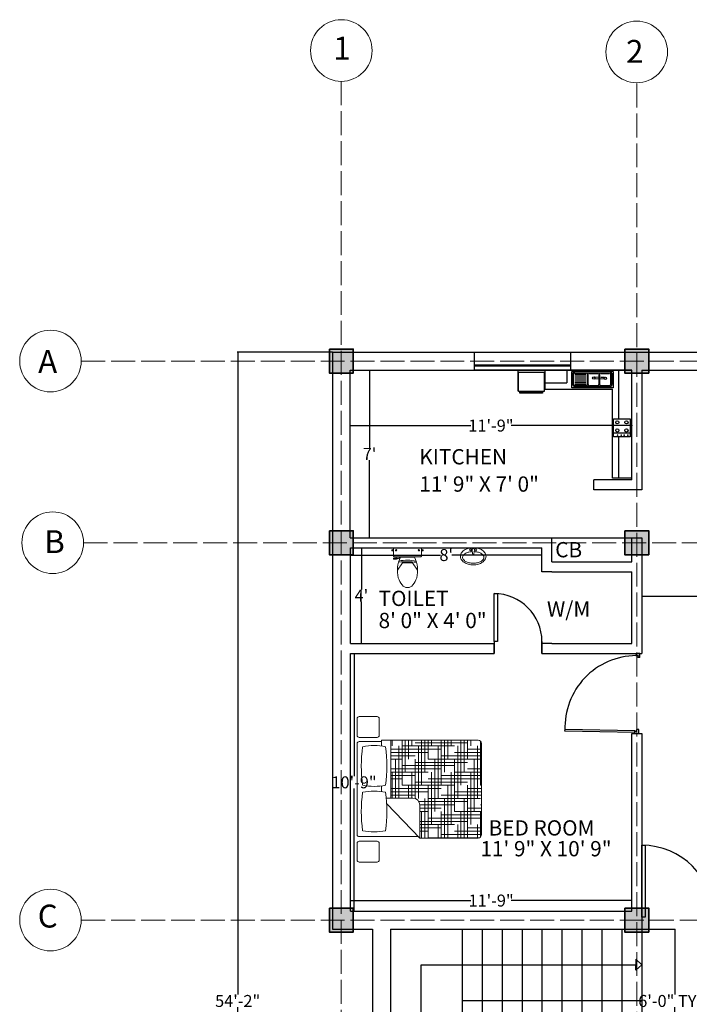
# Model space of a CAD drawing. Units: inches. Extents: x -113 to 5399, y -1393 to 3302.
# Tile 6 of 40: x 737 to 1073, y 460 to 953. Entities that reach past the tile are written whole.
import ezdxf

# ---------------------------------------------------------------- set-up
doc = ezdxf.new("R2010")
doc.units = ezdxf.units.IN
doc.header["$MEASUREMENT"] = 0
doc.linetypes.add('ACAD_ISO02W100', pattern=[15, 12, -3])
for name, color, linetype, lineweight in [('A-ANNO-DIMS', 254, 'Continuous', 18), ('A-AREA-IDEN', 4, 'Continuous', 18), ('A-COLS', 7, 'Continuous', 35), ('A-FLOR-CASE', 8, 'Continuous', 18), ('A-FLOR-FIXT', 8, 'Continuous', 18), ('A-GRID-IDEN', 7, 'Continuous', 18), ('doors', 2, 'Continuous', 25), ('DT TEXT', 4, 'Continuous', 18), ('furniture', 131, 'Continuous', 18), ('GRIDS', 7, 'ACAD_ISO02W100', 13), ('stairs', 210, 'Continuous', 25), ('walls', 1, 'Continuous', 25), ('windows', 3, 'Continuous', 25)]:
    doc.layers.add(name, color=color, linetype=linetype, lineweight=lineweight)
doc.layers.add('TEFRIŞ', color=11, linetype='Continuous')
doc.styles.get("Standard").update_dxf_attribs({"font": 'arial.ttf'})
doc.dimstyles.get("Standard").update_dxf_attribs({"dimtxt": 6, "dimasz": 0.18, "dimexe": 0.18, "dimexo": 0.0625, "dimgap": 0.09, "dimtad": 0, "dimtih": 1, "dimtoh": 1, "dimdec": 1, "dimzin": 0, "dimdsep": 46, "dimlunit": 4, "dimtxsty": 'Standard', "dimblk": 'ARCHTICK', "dimcen": 0.09, "dimadec": 0, "dimazin": 0, "dimtfac": 1, "dimtdec": 1, "dimtofl": 0, "dimtmove": 0, "dimatfit": 3, "dimfxl": 1, "dimtolj": 1, "dimtzin": 0, "dimarcsym": 0})

# ---------------------------------------------------------------- blocks, each defined once
blk = doc.blocks.new('*U2')
for p, q in [((0, 0), (0, -6)), ((24, 0), (24, -6))]:
    blk.add_line(p, q)
blk.add_lwpolyline([(0, 0), (0, 24), (1.75, 24), (1.75, 0)], close=True)
blk.add_arc((0, 0), 24, 0, 90)
blk = doc.blocks.new('*U3')
for p, q in [((0, 0), (0, -6)), ((36, 0), (36, -6))]:
    blk.add_line(p, q)
blk.add_lwpolyline([(0, 0), (0, 36), (1.75, 36), (1.75, 0)], close=True)
blk.add_arc((0, 0), 36, 0, 90)
blk = doc.blocks.new('*X4')
at = {"color": 0}
for p, q in [((4.359, 18.562), (4.359, 18.646)), ((4.5, 18), (4.5, 18.646)), ((4.547, 18.188), (4.547, 18.646)), ((4.594, 18.375), (4.594, 18.646)), ((4.641, 18.562), (4.641, 18.646)), ((4.687, 18.609), (5.437, 18.609)), ((4.781, 18), (4.781, 18.646)), ((4.828, 18.188), (4.828, 18.646)), ((4.875, 18.375), (4.875, 18.646)), ((4.922, 18.562), (4.922, 18.646)), ((5.062, 18), (5.062, 18.646)), ((5.109, 18.188), (5.109, 18.646)), ((5.156, 18.375), (5.156, 18.646)), ((5.203, 18.562), (5.203, 18.646)), ((5.344, 18), (5.344, 18.646)), ((5.391, 18.188), (5.391, 18.646)), ((5.437, 18.375), (5.437, 18.646)), ((5.484, 18.562), (5.484, 18.646)), ((5.625, 18), (5.625, 18.629)), ((4.34, 18.516), (5.062, 18.516)), ((4.34, 18.469), (4.875, 18.469)), ((4.453, 17.817), (4.453, 18.562)), ((4.5, 18.562), (5.25, 18.562)), ((4.734, 17.812), (4.734, 18.562)), ((5.016, 17.812), (5.016, 18.562)), ((5.25, 18.469), (5.637, 18.469)), ((5.297, 17.812), (5.297, 18.562)), ((5.437, 18.516), (5.637, 18.516)), ((5.578, 17.812), (5.578, 18.562)), ((5.625, 18.562), (5.637, 18.562)), ((4.34, 18.422), (4.687, 18.422)), ((4.34, 18.375), (4.5, 18.375)), ((4.406, 17.817), (4.406, 18.375)), ((4.687, 18.328), (5.437, 18.328)), ((4.687, 17.811), (4.687, 18.375)), ((4.875, 18.375), (5.625, 18.375)), ((4.969, 17.625), (4.969, 18.375)), ((5.062, 18.422), (5.637, 18.422)), ((5.25, 17.625), (5.25, 18.375)), ((5.531, 17.625), (5.531, 18.375)), ((4.34, 18.234), (5.062, 18.234)), ((4.34, 18.188), (4.875, 18.188)), ((4.359, 17.817), (4.359, 18.188)), ((4.5, 18.281), (5.25, 18.281)), ((4.641, 17.817), (4.641, 18.188)), ((4.922, 17.438), (4.922, 18.188)), ((5.203, 17.438), (5.203, 18.188)), ((5.25, 18.188), (5.637, 18.188)), ((5.437, 18.234), (5.637, 18.234)), ((5.484, 17.438), (5.484, 18.188)), ((5.625, 18.281), (5.637, 18.281)), ((4.34, 18.141), (4.687, 18.141)), ((4.34, 18.094), (4.5, 18.094)), ((4.687, 18.047), (5.437, 18.047)), ((4.875, 18.094), (5.625, 18.094)), ((5.062, 18.141), (5.637, 18.141)), ((4.34, 17.953), (5.062, 17.953)), ((4.34, 17.906), (4.875, 17.906)), ((4.5, 18), (5.25, 18)), ((4.594, 17.817), (4.594, 18)), ((4.875, 17.25), (4.875, 18)), ((5.156, 17.25), (5.156, 18)), ((5.25, 17.906), (5.637, 17.906)), ((5.437, 17.953), (5.637, 17.953)), ((5.437, 17.25), (5.437, 18)), ((5.625, 18), (5.637, 18)), ((4.34, 17.859), (4.687, 17.859)), ((4.742, 17.766), (5.437, 17.766)), ((4.828, 17.246), (4.828, 17.812)), ((4.875, 17.812), (5.625, 17.812)), ((5.062, 17.859), (5.637, 17.859)), ((5.109, 17.246), (5.109, 17.812)), ((5.391, 17.246), (5.391, 17.812)), ((4.755, 17.719), (5.25, 17.719)), ((4.755, 17.672), (5.062, 17.672)), ((4.755, 17.625), (4.875, 17.625)), ((4.781, 17.246), (4.781, 17.625)), ((5.062, 17.246), (5.062, 17.625)), ((5.25, 17.625), (5.637, 17.625)), ((5.344, 17.246), (5.344, 17.625)), ((5.437, 17.672), (5.637, 17.672)), ((5.625, 17.719), (5.637, 17.719)), ((5.625, 17.263), (5.625, 17.625)), ((4.755, 17.484), (5.437, 17.484)), ((4.875, 17.531), (5.625, 17.531)), ((5.062, 17.578), (5.637, 17.578)), ((4.755, 17.438), (5.25, 17.438)), ((4.755, 17.391), (5.062, 17.391)), ((4.755, 17.344), (4.875, 17.344)), ((5.016, 17.246), (5.016, 17.438)), ((5.25, 17.344), (5.637, 17.344)), ((5.297, 17.246), (5.297, 17.438)), ((5.437, 17.391), (5.637, 17.391)), ((5.578, 17.246), (5.578, 17.438)), ((5.625, 17.438), (5.637, 17.438)), ((4.875, 17.25), (5.608, 17.25)), ((4.969, 17.246), (4.969, 17.25)), ((5.062, 17.297), (5.637, 17.297)), ((5.25, 17.246), (5.25, 17.25)), ((5.531, 17.246), (5.531, 17.25))]:
    blk.add_line(p, q, dxfattribs=at)
blk = doc.blocks.new('MAT-P01')
for p, q in [((0.009, 0.846), (0.247, 0.846)), ((0.374, 0.846), (1.674, 0.846)), ((1.792, 0.846), (2.031, 0.846)), ((-0.021, 0.816), (-0.021, 0.56)), ((0.277, 0.816), (0.277, 0.56)), ((0.344, 0.816), (0.344, -0.032)), ((1.704, 0.816), (1.704, 0.5)), ((1.762, 0.816), (1.762, 0.56)), ((2.061, 0.816), (2.061, 0.56)), ((0.009, 0.53), (0.247, 0.53)), ((0.815, 0.423), (0.324, -0.051)), ((0.895, 0.429), (0.895, 0.049)), ((0.988, 0.5), (1.069, 0.5)), ((1.639, 0.5), (1.724, 0.5)), ((1.724, 0.5), (1.724, -0.884)), ((1.792, 0.53), (2.031, 0.53)), ((0.895, 0.364), (1.724, 0.364)), ((0.895, 0.364), (0.895, 0.049)), ((0.895, 0.364), (1.724, 0.364)), ((1.724, 0.364), (1.724, -0.884)), ((0.324, -0.051), (0.795, -0.051)), ((0.324, -0.051), (0.324, -0.884)), ((0.374, -0.934), (1.674, -0.934))]:
    blk.add_line(p, q)
for centre, radius, start, end in [((0.009, 0.816), 0.03, 90, 180), ((0.247, 0.816), 0.03, 0, 90), ((0.374, 0.816), 0.03, 90, 180), ((1.674, 0.816), 0.03, 0, 90), ((1.792, 0.816), 0.03, 90, 180), ((2.031, 0.816), 0.03, 0, 90), ((1.225, 0.603), 0.814, 168.373, 191.627), ((0.703, -1.144), 1.931, 81.8162, 98.1838), ((0.181, 0.603), 0.814, 348.373, 11.627), ((1.877, 0.603), 0.814, 168.373, 191.627), ((1.354, -1.144), 1.931, 81.8162, 98.1838), ((0.832, 0.603), 0.814, 348.373, 11.627), ((0.009, 0.56), 0.03, 180, 270), ((0.247, 0.56), 0.03, 270, 0), ((0.703, 2.35), 1.931, 261.8162, 278.1838), ((1.354, 2.35), 1.931, 261.8162, 278.1838), ((1.792, 0.56), 0.03, 180, 270), ((2.031, 0.56), 0.03, 270, 0), ((0.795, 0.049), 0.1, 270, 0), ((0.374, -0.884), 0.05, 180, 270), ((1.674, -0.884), 0.05, 270, 0)]:
    blk.add_arc(centre, radius, start, end)
at = {"rotation": 270}
blk.add_blockref('*X4', (-16.922, 4.704), dxfattribs=at)
blk = doc.blocks.new('toilet-3')
at = {"color": 0, "linetype": 'ByBlock'}
for p, q in [((-0.281, -0.05), (-0.281, -0.069)), ((-0.281, -0.05), (-0.261, -0.05)), ((-0.281, -0.069), (-0.261, -0.069)), ((-0.261, -0.047), (-0.261, -0.072)), ((-0.261, -0.047), (-0.251, -0.047)), ((-0.261, -0.072), (-0.251, -0.072)), ((-0.251, -0.047), (-0.251, -0.072)), ((-0.25, -0.03), (-0.25, -0.165)), ((0.24, -0.02), (-0.24, -0.02)), ((0.24, -0.175), (-0.24, -0.175)), ((-0.202, -0.2), (-0.202, -0.175)), ((-0.144, -0.2), (-0.144, -0.175)), ((0.25, -0.03), (0.25, -0.165)), ((0.261, -0.047), (0.251, -0.047)), ((0.251, -0.047), (0.251, -0.072)), ((0.261, -0.072), (0.251, -0.072)), ((0.261, -0.047), (0.261, -0.072)), ((0.281, -0.05), (0.261, -0.05)), ((0.281, -0.069), (0.261, -0.069)), ((0.281, -0.05), (0.281, -0.069)), ((-0.144, -0.2), (-0.25, -0.2)), ((-0.25, -0.2), (-0.25, -0.222)), ((-0.198, -0.222), (-0.25, -0.222)), ((-0.198, -0.222), (-0.16, -0.207)), ((-0.089, -0.287), (-0.18, -0.415)), ((-0.16, -0.207), (-0.16, -0.2)), ((0.125, -0.182), (-0.125, -0.182)), ((0.089, -0.287), (-0.089, -0.287)), ((0.089, -0.287), (0.18, -0.415))]:
    blk.add_line(p, q, dxfattribs=at)
for centre in [(-0.205, -0.059), (0.205, -0.059)]:
    blk.add_circle(centre, 0.0125, dxfattribs=at)
for centre, radius, start, end in [((-0.24, -0.03), 0.01, 90, 180), ((-0.24, -0.165), 0.01, 180, 270), ((0.24, -0.03), 0.01, 0, 90), ((0.24, -0.165), 0.01, 270, 0), ((0.376, -0.424), 0.557, 154.2321, 193.6755), ((-0.013, -1.787), 1.521, 83.4552, 95.5271), ((-0.005, -0.896), 0.659, 75.9276, 103.0204), ((-0.376, -0.424), 0.557, 346.3245, 25.7679), ((0.262, -0.406), 0.452, 199.2942, 217.2549), ((-0.001, -0.609), 0.12, 216.3794, 323.6206), ((-0.265, -0.4), 0.457, 322.2382, 340.1051)]:
    blk.add_arc(centre, radius, start, end, dxfattribs=at)
blk = doc.blocks.new('wash-6')
at = {"color": 0, "linetype": 'ByBlock'}
for p, q in [((-0.036, -0.063), (-0.021, -0.18)), ((0.036, -0.063), (0.021, -0.18))]:
    blk.add_line(p, q, dxfattribs=at)
for centre, radius in [((-0.075, -0.062), 0.0325), ((-0.075, -0.062), 0.0263), ((0.075, -0.062), 0.0325), ((0.075, -0.062), 0.0263)]:
    blk.add_circle(centre, radius, dxfattribs=at)
for centre, radius, start, end in [((0, -0.56), 0.56, 90, 105.4371), ((-0.204, -0.25), 0.17, 148.1465, 180), ((-0.204, -0.25), 0.17, 180, 211.8535), ((-0.107, -0.311), 0.285, 123.6901, 148.1465), ((-0.217, -0.282), 0.0954, 142.5096, 180), ((-0.217, -0.282), 0.0954, 180, 217.4904), ((-0.114, -0.361), 0.225, 118.369, 142.5096), ((-0.042, -0.407), 0.401, 105.4371, 123.6901), ((-0.045, -0.488), 0.37, 102.6081, 118.369), ((0, -0.69), 0.576, 92.9466, 102.6081), ((0, -0.063), 0.0361, 0, 180), ((0, -0.18), 0.0215, 180, 0), ((0, -0.56), 0.56, 74.5629, 90), ((0, -0.69), 0.576, 77.3919, 87.0534), ((0.045, -0.488), 0.37, 61.631, 77.3919), ((0.042, -0.407), 0.401, 56.3099, 74.5629), ((0.114, -0.361), 0.225, 37.4904, 61.631), ((0.107, -0.311), 0.285, 31.8535, 56.3099), ((0.217, -0.282), 0.0954, 0, 37.4904), ((0.217, -0.282), 0.0954, 322.5096, 0), ((0.204, -0.25), 0.17, 0, 31.8535), ((0.204, -0.25), 0.17, 328.1465, 0), ((-0.107, -0.189), 0.285, 211.8535, 236.3099), ((-0.114, -0.203), 0.225, 217.4904, 241.631), ((-0.042, -0.092), 0.401, 236.3099, 254.5629), ((-0.045, -0.076), 0.37, 241.631, 257.3919), ((0, 0.06), 0.56, 254.5629, 270), ((0, 0.125), 0.576, 257.3919, 270), ((0, 0.125), 0.576, 270, 282.6081), ((0, 0.06), 0.56, 270, 285.4371), ((0.045, -0.076), 0.37, 282.6081, 298.369), ((0.042, -0.092), 0.401, 285.4371, 303.6901), ((0.114, -0.203), 0.225, 298.369, 322.5096), ((0.107, -0.189), 0.285, 303.6901, 328.1465)]:
    blk.add_arc(centre, radius, start, end, dxfattribs=at)
blk = doc.blocks.new('_ArchTick')
at = {"color": 0, "linetype": 'ByBlock', "const_width": 0.15}
blk.add_lwpolyline([(-0.5, -0.5), (0.5, 0.5)], dxfattribs=at)
blk = doc.blocks.new('*D22')
at = {"layer": 'A-ANNO-DIMS', "color": 0, "lineweight": -2, "transparency": 16777216}
for p, q in [((894.17, 786.53), (846.52, 786.53)), ((846.7, 786.53), (846.7, 464.69)), ((846.7, 136.53), (846.7, 458.38)), ((894.17, 136.53), (846.52, 136.53))]:
    blk.add_line(p, q, dxfattribs=at)
at = {"layer": 'Defpoints', "color": 0, "transparency": 16777216}
for p in [(894.23, 786.53), (846.7, 136.53), (894.23, 136.53)]:
    blk.add_point(p, dxfattribs=at)
at = {"layer": 'A-ANNO-DIMS', "color": 0, "lineweight": -2, "transparency": 16777216, "xscale": 0.18, "yscale": 0.18, "zscale": 0.18}
for p, rotation in [((846.7, 786.53), 90), ((846.7, 136.53), 270)]:
    blk.add_blockref('_ArchTick', p, dxfattribs=dict(at, rotation=rotation))
at = {"layer": 'A-ANNO-DIMS', "color": 0, "transparency": 16777216, "insert": (846.7, 461.53), "char_height": 6, "attachment_point": 5}
blk.add_mtext('\\A1;54\'-2"', dxfattribs=at)
blk = doc.blocks.new('*D23')
at = {"layer": 'A-ANNO-DIMS', "color": 0, "lineweight": -2, "transparency": 16777216}
for p, q in [((903.08, 749.97), (903.08, 749.51)), ((903.08, 749.69), (963.54, 749.69)), ((1044.23, 749.69), (983.77, 749.69)), ((1044.23, 749.97), (1044.23, 749.51))]:
    blk.add_line(p, q, dxfattribs=at)
at = {"layer": 'Defpoints', "color": 0, "transparency": 16777216}
for p in [(903.08, 750.03), (903.08, 749.69), (1044.23, 750.03)]:
    blk.add_point(p, dxfattribs=at)
at = {"layer": 'A-ANNO-DIMS', "color": 0, "lineweight": -2, "transparency": 16777216, "xscale": 0.18, "yscale": 0.18, "zscale": 0.18, "rotation": 180}
blk.add_blockref('_ArchTick', (903.08, 749.69), dxfattribs=at)
at = {"layer": 'A-ANNO-DIMS', "color": 0, "lineweight": -2, "transparency": 16777216, "xscale": 0.18, "yscale": 0.18, "zscale": 0.18}
blk.add_blockref('_ArchTick', (1044.23, 749.69), dxfattribs=at)
at = {"layer": 'A-ANNO-DIMS', "color": 0, "transparency": 16777216, "insert": (973.65, 749.69), "char_height": 6, "attachment_point": 5}
blk.add_mtext('\\A1;11\'-9"', dxfattribs=at)
blk = doc.blocks.new('*D24')
at = {"layer": 'A-ANNO-DIMS', "color": 0, "lineweight": -2, "transparency": 16777216}
for p, q in [((912.78, 777.53), (912.78, 738.62)), ((912.82, 777.53), (912.96, 777.53)), ((912.78, 693.53), (912.78, 732.44)), ((912.82, 693.53), (912.96, 693.53))]:
    blk.add_line(p, q, dxfattribs=at)
at = {"layer": 'Defpoints', "color": 0, "transparency": 16777216}
for p in [(912.75, 777.53), (912.75, 693.53), (912.78, 693.53)]:
    blk.add_point(p, dxfattribs=at)
at = {"layer": 'A-ANNO-DIMS', "color": 0, "lineweight": -2, "transparency": 16777216, "xscale": 0.18, "yscale": 0.18, "zscale": 0.18}
for p, rotation in [((912.78, 777.53), 90), ((912.78, 693.53), 270)]:
    blk.add_blockref('_ArchTick', p, dxfattribs=dict(at, rotation=rotation))
at = {"layer": 'A-ANNO-DIMS', "color": 0, "transparency": 16777216, "insert": (912.78, 735.53), "char_height": 6, "attachment_point": 5}
blk.add_mtext("\\A1;7'", dxfattribs=at)
blk = doc.blocks.new('*D26')
at = {"layer": 'A-ANNO-DIMS', "color": 0, "lineweight": -2, "transparency": 16777216}
for p, q in [((1049.23, 664.47), (1049.23, 664.12)), ((1049.23, 664.3), (1110.33, 664.3)), ((1181.23, 664.3), (1120.13, 664.3)), ((1181.23, 664.47), (1181.23, 664.12))]:
    blk.add_line(p, q, dxfattribs=at)
at = {"layer": 'Defpoints', "color": 0, "transparency": 16777216}
for p in [(1049.23, 664.53), (1181.23, 664.53), (1181.23, 664.3)]:
    blk.add_point(p, dxfattribs=at)
at = {"layer": 'A-ANNO-DIMS', "color": 0, "lineweight": -2, "transparency": 16777216, "xscale": 0.18, "yscale": 0.18, "zscale": 0.18, "rotation": 180}
blk.add_blockref('_ArchTick', (1049.23, 664.3), dxfattribs=at)
at = {"layer": 'A-ANNO-DIMS', "color": 0, "lineweight": -2, "transparency": 16777216, "xscale": 0.18, "yscale": 0.18, "zscale": 0.18}
blk.add_blockref('_ArchTick', (1181.23, 664.3), dxfattribs=at)
at = {"layer": 'A-ANNO-DIMS', "color": 0, "transparency": 16777216, "insert": (1115.23, 664.3), "char_height": 6, "attachment_point": 5}
blk.add_mtext("\\A1;11'", dxfattribs=at)
blk = doc.blocks.new('*D29')
at = {"layer": 'A-ANNO-DIMS', "color": 0, "lineweight": -2, "transparency": 16777216}
for p, q in [((907.92, 688.53), (908.9, 688.53)), ((908.72, 688.53), (908.72, 667.62)), ((908.72, 640.53), (908.72, 661.44)), ((907.92, 640.53), (908.9, 640.53))]:
    blk.add_line(p, q, dxfattribs=at)
at = {"layer": 'Defpoints', "color": 0, "transparency": 16777216}
for p in [(907.86, 688.53), (907.86, 640.53), (908.72, 640.53)]:
    blk.add_point(p, dxfattribs=at)
at = {"layer": 'A-ANNO-DIMS', "color": 0, "lineweight": -2, "transparency": 16777216, "xscale": 0.18, "yscale": 0.18, "zscale": 0.18}
for p, rotation in [((908.72, 688.53), 90), ((908.72, 640.53), 270)]:
    blk.add_blockref('_ArchTick', p, dxfattribs=dict(at, rotation=rotation))
at = {"layer": 'A-ANNO-DIMS', "color": 0, "transparency": 16777216, "insert": (908.72, 664.53), "char_height": 6, "attachment_point": 5}
blk.add_mtext("\\A1;4'", dxfattribs=at)
blk = doc.blocks.new('*D30')
at = {"layer": 'A-ANNO-DIMS', "color": 0, "lineweight": -2, "transparency": 16777216}
for p, q in [((903.23, 684.92), (903.23, 685.04)), ((903.23, 684.86), (948.38, 684.86)), ((999.23, 684.86), (954.09, 684.86)), ((999.23, 684.92), (999.23, 685.04))]:
    blk.add_line(p, q, dxfattribs=at)
at = {"layer": 'Defpoints', "color": 0, "transparency": 16777216}
for p in [(903.23, 684.86), (999.23, 684.86), (999.23, 684.86)]:
    blk.add_point(p, dxfattribs=at)
at = {"layer": 'A-ANNO-DIMS', "color": 0, "lineweight": -2, "transparency": 16777216, "xscale": 0.18, "yscale": 0.18, "zscale": 0.18, "rotation": 180}
blk.add_blockref('_ArchTick', (903.23, 684.86), dxfattribs=at)
at = {"layer": 'A-ANNO-DIMS', "color": 0, "lineweight": -2, "transparency": 16777216, "xscale": 0.18, "yscale": 0.18, "zscale": 0.18}
blk.add_blockref('_ArchTick', (999.23, 684.86), dxfattribs=at)
at = {"layer": 'A-ANNO-DIMS', "color": 0, "transparency": 16777216, "insert": (951.23, 684.86), "char_height": 6, "attachment_point": 5}
blk.add_mtext("\\A1;8'", dxfattribs=at)
blk = doc.blocks.new('*D31')
at = {"layer": 'A-ANNO-DIMS', "color": 0, "lineweight": -2, "transparency": 16777216}
for p, q in [((905.02, 635.53), (905.02, 574.19)), ((905.08, 635.53), (905.2, 635.53)), ((905.02, 506.53), (905.02, 567.88)), ((905.08, 506.53), (905.2, 506.53))]:
    blk.add_line(p, q, dxfattribs=at)
at = {"layer": 'Defpoints', "color": 0, "transparency": 16777216}
for p in [(905.02, 635.53), (905.02, 506.53), (905.02, 506.53)]:
    blk.add_point(p, dxfattribs=at)
at = {"layer": 'A-ANNO-DIMS', "color": 0, "lineweight": -2, "transparency": 16777216, "xscale": 0.18, "yscale": 0.18, "zscale": 0.18}
for p, rotation in [((905.02, 635.53), 90), ((905.02, 506.53), 270)]:
    blk.add_blockref('_ArchTick', p, dxfattribs=dict(at, rotation=rotation))
at = {"layer": 'A-ANNO-DIMS', "color": 0, "transparency": 16777216, "insert": (905.02, 571.03), "char_height": 6, "attachment_point": 5}
blk.add_mtext('\\A1;10\'-9"', dxfattribs=at)
blk = doc.blocks.new('*D32')
at = {"layer": 'A-ANNO-DIMS', "color": 0, "lineweight": -2, "transparency": 16777216}
for p, q in [((903.23, 511.33), (903.23, 512)), ((903.23, 511.82), (963.62, 511.82)), ((1044.23, 511.82), (983.84, 511.82)), ((1044.23, 511.33), (1044.23, 512))]:
    blk.add_line(p, q, dxfattribs=at)
at = {"layer": 'Defpoints', "color": 0, "transparency": 16777216}
for p in [(903.23, 511.26), (1044.23, 511.82), (1044.23, 511.26)]:
    blk.add_point(p, dxfattribs=at)
at = {"layer": 'A-ANNO-DIMS', "color": 0, "lineweight": -2, "transparency": 16777216, "xscale": 0.18, "yscale": 0.18, "zscale": 0.18, "rotation": 180}
blk.add_blockref('_ArchTick', (903.23, 511.82), dxfattribs=at)
at = {"layer": 'A-ANNO-DIMS', "color": 0, "lineweight": -2, "transparency": 16777216, "xscale": 0.18, "yscale": 0.18, "zscale": 0.18}
blk.add_blockref('_ArchTick', (1044.23, 511.82), dxfattribs=at)
at = {"layer": 'A-ANNO-DIMS', "color": 0, "transparency": 16777216, "insert": (973.73, 511.82), "char_height": 6, "attachment_point": 5}
blk.add_mtext('\\A1;11\'-9"', dxfattribs=at)
blk = doc.blocks.new('A$C008029BD')
at = {"layer": 'TEFRIŞ', "ltscale": 0.05}
for p, q in [((0, 0), (0, -3.55)), ((3.37, 0), (0, 0)), ((3.37, 0), (3.37, -0.6)), ((1.522, -0.4), (0, -0.4)), ((0.05, -0.581), (0.05, -1.869)), ((0.05, -0.581), (0.55, -0.581)), ((0.55, -0.581), (0.55, -1.869)), ((0.6, -2.71), (0.6, -0.6)), ((3.37, -0.6), (0.6, -0.6)), ((3.37, -0.4), (2.083, -0.4)), ((0.086, -1.773), (0.086, -0.677)), ((0.096, -0.617), (0.454, -0.617)), ((0.099, -0.659), (0.457, -0.659)), ((0.113, -0.954), (0.113, -0.695)), ((0.23, -0.846), (0.229, -0.967)), ((0.28, -0.846), (0.277, -1.158)), ((0.493, -0.695), (0.493, -0.954)), ((0.514, -0.677), (0.514, -1.773)), ((0.096, -1.024), (0.454, -1.024)), ((0.457, -0.99), (0.099, -0.99)), ((0.11, -1.319), (0.11, -1.06)), ((0.228, -1.02), (0.227, -1.159)), ((0.49, -1.06), (0.49, -1.319)), ((0.454, -1.355), (0.096, -1.355)), ((0.096, -1.391), (0.454, -1.391)), ((0.11, -1.773), (0.11, -1.427)), ((0.154, -1.773), (0.154, -1.427)), ((0.214, -1.773), (0.214, -1.427)), ((0.274, -1.773), (0.274, -1.427)), ((0.334, -1.773), (0.334, -1.427)), ((0.39, -1.773), (0.39, -1.427)), ((0.444, -1.773), (0.444, -1.427)), ((0.49, -1.427), (0.49, -1.773)), ((0.454, -1.809), (0.096, -1.809)), ((0.454, -1.833), (0.096, -1.833)), ((0, -2.025), (0.4, -2.025)), ((0.55, -1.869), (0.05, -1.869)), ((0.4, -2.71), (0.4, -2.025)), ((0, -2.71), (0.6, -2.71)), ((0, -3.55), (0.65, -3.55))]:
    blk.add_line(p, q, dxfattribs=at)
at = {"layer": 'TEFRIŞ'}
blk.add_line((1.969, -0.05), (1.969, -0.572), dxfattribs=at)
at = {"layer": 'TEFRIŞ', "ltscale": 0.05}
for points in [[(1.522, -0.05), (2.083, -0.05), (2.083, -0.572), (1.522, -0.572)], [(0.67, -2.73), (0.67, -3.53), (0.07, -3.53), (0.07, -2.73)], [(0.72, -2.78), (0.72, -3.48), (0.67, -3.48), (0.67, -2.78)]]:
    blk.add_lwpolyline(points, close=True, dxfattribs=at)
at = {"layer": 'TEFRIŞ', "const_width": 0.025}
for points in [[(2.014, -0.123, 1), (2.039, -0.123, 1)], [(2.014, -0.236, 1), (2.039, -0.236, 1)], [(2.014, -0.327, 1), (2.039, -0.327, 1)], [(2.014, -0.44, 1), (2.039, -0.44, 1)]]:
    blk.add_lwpolyline(points, format="xyb", close=True, dxfattribs=at)
at = {"layer": 'TEFRIŞ', "ltscale": 0.05}
for centre, radius in [((1.628, -0.164), 0.0505), ((1.628, -0.45), 0.0505), ((0.255, -0.82), 0.036), ((0.252, -1.184), 0.036)]:
    blk.add_circle(centre, radius, dxfattribs=at)
at = {"layer": 'TEFRIŞ'}
for centre in [(1.88, -0.164), (1.88, -0.45)]:
    blk.add_circle(centre, 0.0505, dxfattribs=at)
at = {"layer": 'TEFRIŞ', "ltscale": 0.05}
for centre, radius, start, end in [((0.108, -0.649), 0.0351, 110.4976, 230.5777), ((0.118, -0.673), 0.023, 143.9853, 258.5157), ((0.454, -0.677), 0.06, 0, 90), ((0.457, -0.695), 0.036, 0, 90), ((0.115, -1.038), 0.023, 143.9853, 258.5157), ((0.118, -0.976), 0.023, 101.4843, 216.0147), ((0.454, -1.06), 0.036, 0, 90), ((0.457, -0.954), 0.036, 270, 0), ((0.115, -1.341), 0.023, 101.4843, 216.0147), ((0.115, -1.405), 0.023, 143.9853, 258.5157), ((0.454, -1.319), 0.036, 270, 0), ((0.454, -1.427), 0.036, 0, 90), ((0.108, -1.801), 0.0351, 129.4223, 249.5024), ((0.115, -1.796), 0.023, 101.4843, 216.0147), ((0.454, -1.773), 0.06, 270, 0), ((0.454, -1.773), 0.036, 270, 0)]:
    blk.add_arc(centre, radius, start, end, dxfattribs=at)
blk = doc.blocks.new('WIN-PLAN-48IN')
h = blk.add_hatch(color=256)
h.dxf.hatch_style = 1
h.paths.add_polyline_path([(48, 2.5), (0, 2.5), (0, 2), (48, 2)])
for p, q in [((0, 9), (48, 9)), ((0, 0), (0, 9)), ((48, 9), (48, 0)), ((48, 2.5), (0, 2.5)), ((48, 2), (0, 2)), ((48, 0), (0, 0))]:
    blk.add_line(p, q)
blk = doc.blocks.new('COLUMN-12IN-SQUARE')
h = blk.add_hatch(color=256)
h.dxf.hatch_style = 1
h.paths.add_polyline_path([(6, 6), (-6, 6), (-6, -6), (6, -6)])
blk.add_lwpolyline([(-6, 6), (6, 6), (6, -6), (-6, -6)], close=True)
blk = doc.blocks.new('STAIR-RESIDENTIAL-PLAN')
for p, q in [((20.54, 72), (20.54, 0)), ((30.54, 72), (30.54, 0)), ((40.54, 72), (40.54, 0)), ((50.54, 72), (50.54, 0)), ((60.54, 72), (60.54, 0)), ((70.54, 72), (70.54, 0)), ((80.54, 72), (80.54, 0)), ((90.54, 72), (90.54, 0)), ((100.54, 72), (100.54, 0)), ((110.54, 72), (110.54, 0)), ((110.54, 54.14), (107.61, 56.9)), ((107.61, 56.9), (107.61, 54.14)), ((0, 17.09), (0, 54.14)), ((0, 54.14), (107.61, 54.14)), ((110.54, 54.14), (107.61, 51.38)), ((107.61, 51.38), (107.61, 54.14)), ((110.54, 36), (20.54, 36)), ((110.54, 17.09), (0, 17.09))]:
    blk.add_line(p, q)
blk = doc.blocks.new('DOOR-SINGLE-36IN-PLAN')
for p, q in [((0.5, 2), (0.5, 36.98)), ((0.5, 36.98), (1.5, 36.98)), ((1.5, 36.98), (1.5, 2)), ((0, 2), (0, 0)), ((0, 2), (1.04, 2)), ((1.5, 2), (0.5, 2)), ((1.04, 2), (1.04, 0.98)), ((1.04, 0.98), (2, 0.98)), ((2, 0), (2, 0.98)), ((38.96, 0.98), (38, 0.98)), ((38, 0), (38, 0.98)), ((40, 2), (38.96, 2)), ((38.96, 2), (38.96, 0.98)), ((40, 0), (40, 2)), ((0, 0), (2, 0)), ((0, 0), (2, 0)), ((38, 0), (40, 0))]:
    blk.add_line(p, q)
blk.add_arc((2.94, 0.99), 36.04, 1.6003, 93.0893)
blk = doc.blocks.new('GRID-BUBBLE-A')
blk.add_circle((0, 0), 15.44)
blk.add_text('A', height=11.45).set_placement((-6.15, -5.94))
blk = doc.blocks.new('GRID-BUBBLE-B')
blk.add_circle((0, 0), 15.44)
blk.add_text('B', height=11.45).set_placement((-4.23, -5.2))
blk = doc.blocks.new('GRID-BUBBLE-C')
blk.add_circle((0, 0), 15.44)
blk.add_text('C', height=11.45).set_placement((-6.38, -3.72))
blk = doc.blocks.new('GRID-BUBBLE-1')
blk.add_circle((0, 0), 15.44)
blk.add_text('1', height=11.45).set_placement((-3.99, -4.52))
blk = doc.blocks.new('GRID-BUBBLE-2')
blk.add_circle((0, 0), 15.44)
blk.add_text('2', height=11.45).set_placement((-5.33, -5.46))
blk = doc.blocks.new('*D194')
at = {"layer": 'A-ANNO-DIMS', "color": 0, "lineweight": -2, "transparency": 16777216}
for p, q in [((1049.29, 497.53), (1065.99, 497.53)), ((1065.81, 497.53), (1065.81, 464.69)), ((1065.81, 425.53), (1065.81, 458.38)), ((1049.29, 425.53), (1065.99, 425.53))]:
    blk.add_line(p, q, dxfattribs=at)
at = {"layer": 'Defpoints', "color": 0, "transparency": 16777216}
for p in [(1049.23, 497.53), (1065.81, 497.53), (1049.23, 425.53)]:
    blk.add_point(p, dxfattribs=at)
at = {"layer": 'A-ANNO-DIMS', "color": 0, "lineweight": -2, "transparency": 16777216, "xscale": 0.18, "yscale": 0.18, "zscale": 0.18}
for p, rotation in [((1065.81, 497.53), 90), ((1065.81, 425.53), 270)]:
    blk.add_blockref('_ArchTick', p, dxfattribs=dict(at, rotation=rotation))
at = {"layer": 'A-ANNO-DIMS', "color": 0, "transparency": 16777216, "insert": (1065.81, 461.53), "char_height": 6, "attachment_point": 5}
blk.add_mtext('\\A1;6\'-0" TYP.', dxfattribs=at)

msp = doc.modelspace()

# ---------------------------------------------------------------- linework, layer by layer
at = {"layer": 'GRIDS'}
for p, q in [((898.65, 922.09), (898.65, 39.31)), ((1046.73, 54.04), (1046.73, 921.39)), ((768.3, 782.03), (1417.18, 782.03)), ((769.42, 691.03), (1426.54, 691.03)), ((768.3, 502.03), (1426.54, 502.03))]:
    msp.add_line(p, q, dxfattribs=at)
at = {"layer": 'walls'}
for p, q in [((894.23, 786.53), (894.23, 497.53)), ((894.23, 786.53), (1091.23, 786.53)), ((903.08, 777.53), (965.48, 777.53)), ((903.08, 693.53), (903.08, 777.53)), ((934.73, 777.53), (1044.23, 777.53)), ((1044.23, 722.53), (1044.23, 777.53)), ((1049.23, 777.53), (1049.23, 717.53)), ((1049.23, 777.53), (1091.23, 777.53)), ((1044.23, 722.53), (1025.23, 722.53)), ((1025.23, 717.53), (1025.23, 722.53)), ((1049.23, 717.53), (1025.23, 717.53)), ((903.08, 693.53), (929.73, 693.53)), ((929.73, 693.53), (934.73, 693.53)), ((934.73, 693.53), (1044.23, 693.53)), ((1004.23, 681.53), (1004.23, 693.53)), ((1044.23, 681.53), (1044.23, 693.53)), ((1044.23, 693.53), (1049.23, 693.53)), ((1049.23, 693.53), (1049.23, 635.53)), ((903.23, 640.53), (903.23, 688.53)), ((903.23, 688.53), (999.23, 688.53)), ((999.23, 676.53), (999.23, 688.53)), ((1004.23, 681.53), (1044.23, 681.53)), ((1004.23, 676.53), (999.23, 676.53)), ((1004.23, 676.53), (1044.23, 676.53)), ((1044.23, 640.53), (1044.23, 676.53)), ((999.23, 635.53), (999.23, 641.53)), ((903.23, 640.53), (975.23, 640.53)), ((975.23, 635.53), (975.23, 640.53)), ((1004.23, 640.53), (999.23, 640.53)), ((1004.23, 640.53), (1044.23, 640.53)), ((903.23, 506.53), (903.23, 635.53)), ((903.23, 635.53), (975.23, 635.53)), ((999.23, 635.53), (1044.23, 635.53)), ((1044.23, 635.53), (1049.23, 635.53)), ((1044.23, 506.53), (1044.23, 595.53)), ((1044.23, 595.53), (1049.23, 595.53)), ((1049.23, 595.53), (1049.23, 506.53)), ((903.23, 506.53), (1044.23, 506.53)), ((1049.23, 506.53), (1049.23, 497.53)), ((894.23, 497.53), (914.23, 497.53)), ((914.23, 497.53), (914.23, 425.53)), ((923.23, 497.53), (1049.23, 497.53)), ((923.23, 497.53), (923.23, 425.53))]:
    msp.add_line(p, q, dxfattribs=at)

# ---------------------------------------------------------------- block references
at = {"layer": 'A-COLS'}
for p in [(898.65, 782.03), (1046.73, 782.03), (898.65, 691.03), (1046.73, 691.03), (898.65, 502.03), (1046.73, 502.03)]:
    msp.add_blockref('COLUMN-12IN-SQUARE', p, dxfattribs=at)
at = {"layer": 'A-FLOR-CASE', "xscale": 16.09806929200166, "yscale": 16.09806929200166, "zscale": 16.09806929200166, "rotation": 270}
msp.add_blockref('A$C008029BD', (1044.23, 777.53), dxfattribs=at)
at = {"layer": 'A-FLOR-FIXT'}
for name, p, xscale, yscale, zscale in [('toilet-3', (931.83, 688.93), 27.95492935005888, 27.95492935005888, 27.95492935005888), ('wash-6', (964.78, 688.53), 17.16666334294967, 17.16666334294967, 17.16666334294967)]:
    msp.add_blockref(name, p, dxfattribs=dict(at, xscale=xscale, yscale=yscale, zscale=zscale))
at = {"layer": 'A-GRID-IDEN'}
for name, p in [('GRID-BUBBLE-1', (898.65, 937.53)), ('GRID-BUBBLE-2', (1046.73, 936.83)), ('GRID-BUBBLE-A', (752.86, 782.03)), ('GRID-BUBBLE-B', (753.98, 691.03)), ('GRID-BUBBLE-C', (752.86, 502.03))]:
    msp.add_blockref(name, p, dxfattribs=at)
at = {"layer": 'doors'}
for name, p in [('*U2', (975.23, 641.53)), ('*U3', (1049.23, 503.53))]:
    msp.add_blockref(name, p, dxfattribs=at)
at = {"layer": 'doors', "rotation": 89.09244041659088}
msp.add_blockref('DOOR-SINGLE-36IN-PLAN', (1047.73, 595.52), dxfattribs=at)
at = {"layer": 'furniture', "xscale": 35.02364872074636, "yscale": 35.02364872074636, "zscale": 35.02364872074636, "rotation": 90}
msp.add_blockref('MAT-P01', (936.22, 531.79), dxfattribs=at)
at = {"layer": 'stairs'}
msp.add_blockref('STAIR-RESIDENTIAL-PLAN', (938.69, 425.53), dxfattribs=at)
at = {"layer": 'windows'}
msp.add_blockref('WIN-PLAN-48IN', (965.48, 777.53), dxfattribs=at)

# ---------------------------------------------------------------- texts
at = {"layer": 'A-AREA-IDEN'}
for s, height, p in [('KITCHEN', 7.647, (937.75, 730.26)), ('11\' 9" X 7\' 0"', 7.6473, (937.75, 716.59)), ('TOILET', 7.647, (917.32, 659.34)), ('8\' 0" X 4\' 0"', 7.6473, (917.32, 648.26)), ('BED ROOM', 7.647, (972.47, 544.39)), ('11\' 9" X 10\' 9"', 7.6473, (968.37, 533.97))]:
    msp.add_text(s, height=height, dxfattribs=at).set_placement(p)
at = {"layer": 'DT TEXT'}
for s, p in [('CB', (1005.85, 683.72)), (' W/M', (999.39, 653.97))]:
    msp.add_text(s, height=7.647, dxfattribs=at).set_placement(p)

# ---------------------------------------------------------------- dimensions: what is measured, and where the dimension line sits
at = {"layer": 'A-ANNO-DIMS'}
for base, p1, p2, picture, middle in [((846.7, 136.53), (894.23, 786.53), (894.23, 136.53), '*D22', (846.7, 461.53)), ((908.72, 640.53), (907.86, 688.53), (907.86, 640.53), '*D29', (908.72, 664.53)), ((905.02, 506.53), (905.02, 635.53), (905.02, 506.53), '*D31', (905.02, 571.03))]:
    dim = msp.add_linear_dim(base=base, p1=p1, p2=p2, angle=90, dimstyle='Standard', override={"dimclrd": 0, "dimclre": 0, "dimclrt": 0}, dxfattribs=at)
    dim.commit()
    dim.dimension.update_dxf_attribs({"geometry": picture, "text_midpoint": middle})
dim = msp.add_linear_dim(base=(912.78, 693.53), p1=(912.75, 777.53), p2=(912.75, 693.53), angle=90, dimstyle='Standard', override={"dimclrd": 0, "dimclre": 0, "dimclrt": 0}, dxfattribs=at)
dim.commit()
dim.dimension.update_dxf_attribs({"geometry": '*D24', "text_midpoint": (912.78, 735.53), "dimtype": 160})
for base, p1, p2, picture, middle in [((903.0766, 749.6912), (1044.2305, 750.032), (903.0766, 750.032), '*D23', (973.6535, 749.6912)), ((999.23, 684.86), (903.23, 684.86), (999.23, 684.86), '*D30', (951.23, 684.86)), ((1181.23, 664.3), (1049.23, 664.53), (1181.23, 664.53), '*D26', (1115.23, 664.3)), ((1044.23, 511.82), (903.23, 511.26), (1044.23, 511.26), '*D32', (973.73, 511.82))]:
    dim = msp.add_linear_dim(base=base, p1=p1, p2=p2, dimstyle='Standard', override={"dimclrd": 0, "dimclre": 0, "dimclrt": 0}, dxfattribs=at)
    dim.commit()
    dim.dimension.update_dxf_attribs({"geometry": picture, "text_midpoint": middle})
dim = msp.add_linear_dim(base=(1065.81, 497.53), p1=(1049.23, 425.53), p2=(1049.23, 497.53), angle=90, text='<> TYP.', dimstyle='Standard', override={"dimdec": 1, "dimlfac": 1, "dimrnd": 0, "dimzin": 1, "dimdsep": 46, "dimlunit": 4, "dimfrac": 2}, dxfattribs=at)
dim.commit()
dim.dimension.update_dxf_attribs({"geometry": '*D194', "text_midpoint": (1065.81, 461.53)})

doc.saveas('drawing.dxf')
